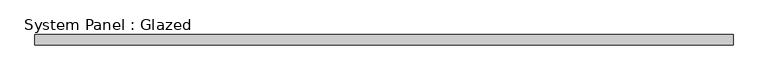
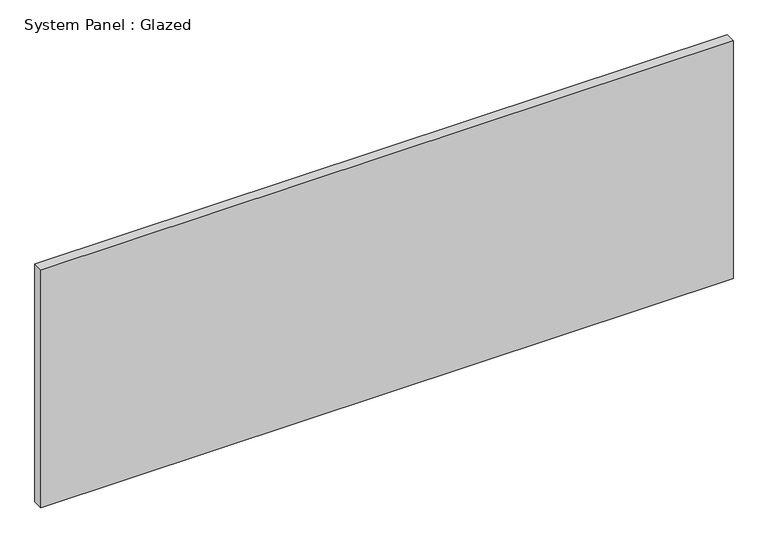
"""IFC4 building model written with IfcOpenShell, lengths in millimetres: plate geometry, System Panel : Glazed."""

from ifc_helpers import new_model, si_unit, origin, origin_with_axes, place, context, project, spatial, polyline, outline, extrude, source, transform, mapped, element, save


def system_panel_glazed_5a474b37(model_context):
    return source(origin(), model_context, "Body", "SweptSolid", [
        extrude(outline(polyline([(838.2, 24.5), (-838.2, 24.5), (-838.2, 49.5), (838.2, 49.5), (838.2, 24.5)])), origin_with_axes(), (0.0, 0.0, 1.0), 609.6),
    ])


if __name__ == "__main__":
    model = new_model("IFC4")
    model_context = context("Model", 3, world=origin())
    ifc_project = project(units=[si_unit("LENGTHUNIT", "METRE", prefix="MILLI")], contexts=[model_context])
    site = spatial("IfcSite", under=ifc_project)
    building = spatial("IfcBuilding", under=site)
    placement = place(None, origin())
    system_panel_glazed_shape = system_panel_glazed_5a474b37(model_context)
    element("IfcPlate", 1, ObjectType="System Panel : Glazed", at=placement, inside=building, context=model_context, shape_type="MappedRepresentation", body=[
        mapped(system_panel_glazed_shape, transform((0.0, 0.0, 0.0), x_axis=(1.0, 0.0, 0.0), y_axis=(0.0, 1.0, 0.0), z_axis=(0.0, 0.0, 1.0))),
    ])
    save(model, "model.ifc")

# Revit data of these elements
# Type "System Panel : Glazed"
#   Keynote = "H11"
#   Construction Type Id = "GSP4R"
#   Analytic Construction = "1/8 in Pilkington single glazing"
#   Visual Light Transmittance = 0.9
#   Solar Heat Gain Coefficient = 0.86
#   Heat Transfer Coefficient (U) = 6.7069 W/(m²·K)
#   Define Thermal Properties by = 1
# Element 1 (IfcPlate, "System Panel : Glazed")
#   Materials on its faces: "Glass"
# Materials
#   "Glass": class "Glass", colour RGB 0 128 192, transparency 0.9, Description = "Soda Lime Glass", Cost = 0
